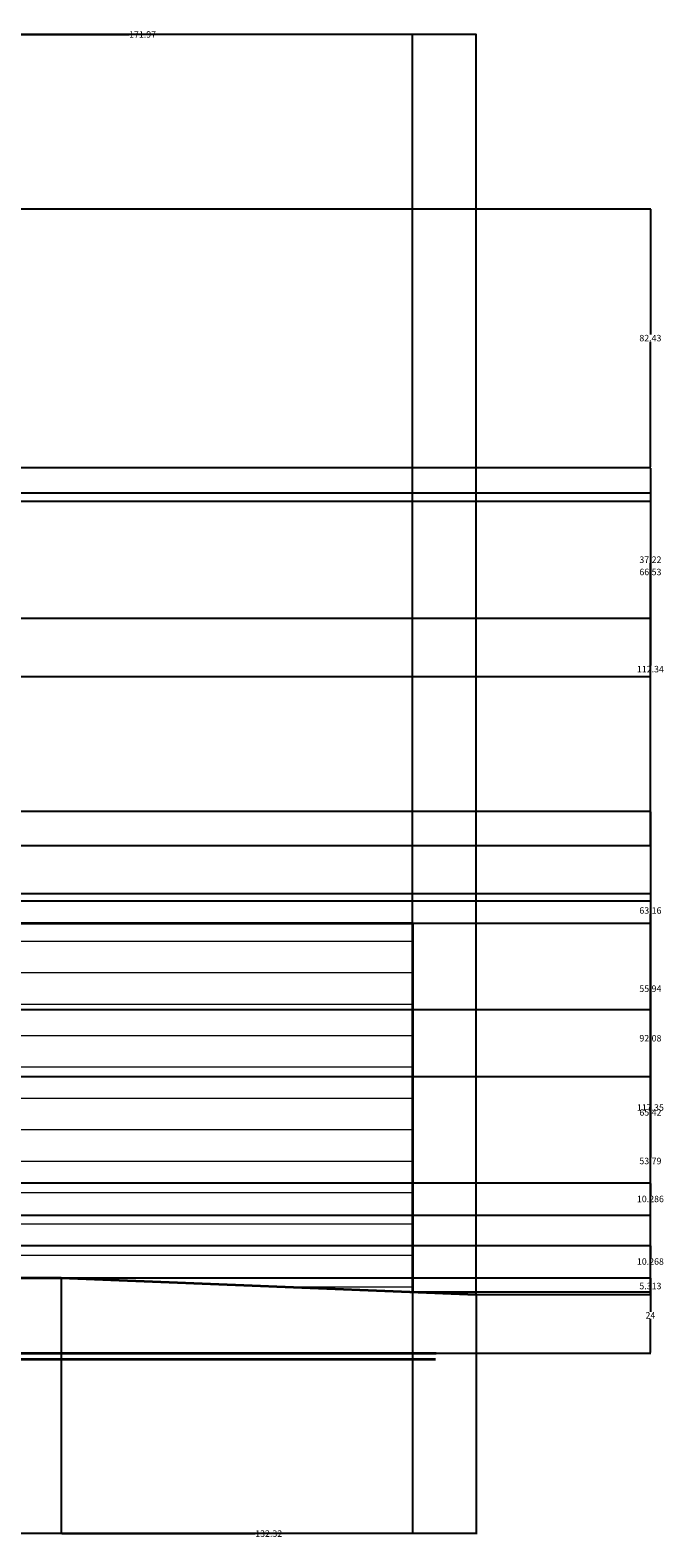
# Model space of a CAD drawing. Units: inches. Extents: x -30 to 1188, y 40 to 520.
# Tile 7 of 7: x 986 to 1188, y 40 to 520. Entities that reach past the tile are written whole.
import ezdxf

# ---------------------------------------------------------------- set-up
doc = ezdxf.new("R2010")
doc.units = ezdxf.units.IN
doc.header["$MEASUREMENT"] = 0
for name, color, linetype, lineweight in [('A-ANNO-DIMS', 2, 'Continuous', 18), ('A-ELEV', 7, 'Continuous', 35), ('A-ELEV-PATT', 8, 'Continuous', 13)]:
    doc.layers.add(name, color=color, linetype=linetype, lineweight=lineweight)
doc.styles.get("Standard").update_dxf_attribs({"font": 'arial.ttf'})
doc.dimstyles.get("Standard").update_dxf_attribs({"dimtxt": 2.0625, "dimasz": 0.18, "dimexe": 0.18, "dimexo": 0.0625, "dimgap": 0.09, "dimtad": 0, "dimtih": 1, "dimtoh": 1, "dimdec": 4, "dimzin": 0, "dimdsep": 46, "dimlunit": 4, "dimtxsty": 'Standard', "dimcen": 0.09, "dimadec": 0, "dimazin": 0, "dimtfac": 1, "dimtdec": 4, "dimtofl": 0, "dimtmove": 0, "dimatfit": 3, "dimfxl": 1, "dimtolj": 1, "dimtzin": 0, "dimarcsym": 0})

# ---------------------------------------------------------------- blocks, each defined once
blk = doc.blocks.new('*D4')
at = {"layer": 'A-ANNO-DIMS', "color": 0, "lineweight": -2, "transparency": 16777216}
for p, q in [((73.66, 122.81), (73.66, 41.19)), ((1107.88, 118.31), (1107.88, 41.19)), ((73.84, 41.37), (586.5, 41.37)), ((1107.7, 41.37), (595.03, 41.37))]:
    blk.add_line(p, q, dxfattribs=at)
at = {"layer": 'A-ANNO-DIMS', "color": 0, "transparency": 16777216}
for points in [[(73.84, 41.4), (73.84, 41.34), (73.66, 41.37)], [(1107.7, 41.4), (1107.7, 41.34), (1107.88, 41.37)]]:
    blk.add_solid(points, dxfattribs=at)
at = {"layer": 'Defpoints', "color": 0, "transparency": 16777216}
for p in [(73.66, 122.87), (1107.88, 118.38), (1107.88, 41.37)]:
    blk.add_point(p, dxfattribs=at)
at = {"layer": 'A-ANNO-DIMS', "color": 0, "transparency": 16777216, "insert": (590.77, 41.37), "char_height": 2.062, "attachment_point": 5}
blk.add_mtext('\\A1;1034.2', dxfattribs=at)
blk = doc.blocks.new('*D8')
at = {"layer": 'A-ANNO-DIMS', "color": 0, "lineweight": -2, "transparency": 16777216}
for p, q in [((935.9, 235.79), (935.9, 518.97)), ((936.08, 518.79), (1017.62, 518.79)), ((1107.7, 518.79), (1026.16, 518.79)), ((1107.88, 235.79), (1107.88, 518.97))]:
    blk.add_line(p, q, dxfattribs=at)
at = {"layer": 'A-ANNO-DIMS', "color": 0, "transparency": 16777216}
for points in [[(936.08, 518.82), (936.08, 518.76), (935.9, 518.79)], [(1107.7, 518.82), (1107.7, 518.76), (1107.88, 518.79)]]:
    blk.add_solid(points, dxfattribs=at)
at = {"layer": 'Defpoints', "color": 0, "transparency": 16777216}
for p in [(1107.88, 518.79), (935.9, 235.73), (1107.88, 235.73)]:
    blk.add_point(p, dxfattribs=at)
at = {"layer": 'A-ANNO-DIMS', "color": 0, "transparency": 16777216, "insert": (1021.89, 518.79), "char_height": 2.062, "attachment_point": 5}
blk.add_mtext('\\A1;171.97', dxfattribs=at)
blk = doc.blocks.new('*D19')
at = {"layer": 'A-ANNO-DIMS', "color": 0, "lineweight": -2, "transparency": 16777216}
for p, q in [((1107.94, 235.73), (1183.93, 235.73)), ((1183.75, 235.55), (1183.75, 178.2)), ((1183.75, 118.56), (1183.75, 175.91)), ((1107.94, 118.38), (1183.93, 118.38))]:
    blk.add_line(p, q, dxfattribs=at)
at = {"layer": 'A-ANNO-DIMS', "color": 0, "transparency": 16777216}
for points in [[(1183.72, 235.55), (1183.78, 235.55), (1183.75, 235.73)], [(1183.72, 118.56), (1183.78, 118.56), (1183.75, 118.38)]]:
    blk.add_solid(points, dxfattribs=at)
at = {"layer": 'Defpoints', "color": 0, "transparency": 16777216}
for p in [(1107.88, 235.73), (1183.75, 235.73), (1107.88, 118.38)]:
    blk.add_point(p, dxfattribs=at)
at = {"layer": 'A-ANNO-DIMS', "color": 0, "transparency": 16777216, "insert": (1183.75, 177.05), "char_height": 2.062, "attachment_point": 5}
blk.add_mtext('\\A1;117.35', dxfattribs=at)
blk = doc.blocks.new('*D23')
at = {"layer": 'A-ANNO-DIMS', "color": 0, "lineweight": -2, "transparency": 16777216}
for p, q in [((980.79, 372.83), (1183.93, 372.83)), ((1183.75, 372.65), (1183.75, 317.8)), ((1183.75, 260.67), (1183.75, 315.52)), ((980.79, 260.49), (1183.93, 260.49))]:
    blk.add_line(p, q, dxfattribs=at)
at = {"layer": 'A-ANNO-DIMS', "color": 0, "transparency": 16777216}
for points in [[(1183.72, 372.65), (1183.78, 372.65), (1183.75, 372.83)], [(1183.72, 260.67), (1183.78, 260.67), (1183.75, 260.49)]]:
    blk.add_solid(points, dxfattribs=at)
at = {"layer": 'Defpoints', "color": 0, "transparency": 16777216}
for p in [(980.73, 372.83), (1183.75, 372.83), (980.73, 260.49)]:
    blk.add_point(p, dxfattribs=at)
at = {"layer": 'A-ANNO-DIMS', "color": 0, "transparency": 16777216, "insert": (1183.75, 316.66), "char_height": 2.062, "attachment_point": 5}
blk.add_mtext('\\A1;112.34', dxfattribs=at)
blk = doc.blocks.new('*D26')
at = {"layer": 'A-ANNO-DIMS', "color": 0, "lineweight": -2, "transparency": 16777216}
for p, q in [((798.37, 380.86), (1183.93, 380.86)), ((1183.75, 380.68), (1183.75, 348.74)), ((1183.75, 314.51), (1183.75, 346.45)), ((798.37, 314.33), (1183.93, 314.33))]:
    blk.add_line(p, q, dxfattribs=at)
at = {"layer": 'A-ANNO-DIMS', "color": 0, "transparency": 16777216}
for points in [[(1183.72, 380.68), (1183.78, 380.68), (1183.75, 380.86)], [(1183.72, 314.51), (1183.78, 314.51), (1183.75, 314.33)]]:
    blk.add_solid(points, dxfattribs=at)
at = {"layer": 'Defpoints', "color": 0, "transparency": 16777216}
for p in [(798.3, 380.86), (1183.75, 380.86), (798.3, 314.33)]:
    blk.add_point(p, dxfattribs=at)
at = {"layer": 'A-ANNO-DIMS', "color": 0, "transparency": 16777216, "insert": (1183.75, 347.6), "char_height": 2.062, "attachment_point": 5}
blk.add_mtext('\\A1;66.53', dxfattribs=at)
blk = doc.blocks.new('*D30')
at = {"layer": 'A-ANNO-DIMS', "color": 0, "lineweight": -2, "transparency": 16777216}
for p, q in [((935.97, 463.29), (1183.93, 463.29)), ((1183.75, 463.11), (1183.75, 423.22)), ((1183.75, 381.04), (1183.75, 420.93)), ((798.37, 380.86), (1183.93, 380.86))]:
    blk.add_line(p, q, dxfattribs=at)
at = {"layer": 'A-ANNO-DIMS', "color": 0, "transparency": 16777216}
for points in [[(1183.72, 463.11), (1183.78, 463.11), (1183.75, 463.29)], [(1183.72, 381.04), (1183.78, 381.04), (1183.75, 380.86)]]:
    blk.add_solid(points, dxfattribs=at)
at = {"layer": 'Defpoints', "color": 0, "transparency": 16777216}
for p in [(935.9, 463.29), (1183.75, 463.29), (798.3, 380.86)]:
    blk.add_point(p, dxfattribs=at)
at = {"layer": 'A-ANNO-DIMS', "color": 0, "transparency": 16777216, "insert": (1183.75, 422.08), "char_height": 2.062, "attachment_point": 5}
blk.add_mtext('\\A1;82.43', dxfattribs=at)
blk = doc.blocks.new('*D35')
at = {"layer": 'A-ANNO-DIMS', "color": 0, "lineweight": -2, "transparency": 16777216}
for p, q in [((99.49, 122.87), (1183.93, 122.87)), ((1183.75, 122.69), (1183.75, 112)), ((1183.75, 99.05), (1183.75, 109.75)), ((99.49, 98.87), (1183.93, 98.87))]:
    blk.add_line(p, q, dxfattribs=at)
at = {"layer": 'A-ANNO-DIMS', "color": 0, "transparency": 16777216}
for points in [[(1183.72, 122.69), (1183.78, 122.69), (1183.75, 122.87)], [(1183.72, 99.05), (1183.78, 99.05), (1183.75, 98.87)]]:
    blk.add_solid(points, dxfattribs=at)
at = {"layer": 'Defpoints', "color": 0, "transparency": 16777216}
for p in [(99.43, 122.87), (1183.75, 122.87), (99.43, 98.87)]:
    blk.add_point(p, dxfattribs=at)
at = {"layer": 'A-ANNO-DIMS', "color": 0, "transparency": 16777216, "insert": (1183.75, 110.87), "char_height": 2.062, "attachment_point": 5}
blk.add_mtext('\\A1;24', dxfattribs=at)
blk = doc.blocks.new('*D36')
at = {"layer": 'A-ANNO-DIMS', "color": 0, "lineweight": -2, "transparency": 16777216}
for p, q in [((99.49, 133.14), (1183.93, 133.14)), ((1183.75, 132.96), (1183.75, 129.15)), ((1183.75, 123.05), (1183.75, 126.86)), ((99.49, 122.87), (1183.93, 122.87))]:
    blk.add_line(p, q, dxfattribs=at)
at = {"layer": 'A-ANNO-DIMS', "color": 0, "transparency": 16777216}
for points in [[(1183.72, 132.96), (1183.78, 132.96), (1183.75, 133.14)], [(1183.72, 123.05), (1183.78, 123.05), (1183.75, 122.87)]]:
    blk.add_solid(points, dxfattribs=at)
at = {"layer": 'Defpoints', "color": 0, "transparency": 16777216}
for p in [(99.43, 133.14), (1183.75, 133.14), (99.43, 122.87)]:
    blk.add_point(p, dxfattribs=at)
at = {"layer": 'A-ANNO-DIMS', "color": 0, "transparency": 16777216, "insert": (1183.75, 128.01), "char_height": 2.062, "attachment_point": 5}
blk.add_mtext('\\A1;10.268', dxfattribs=at)
blk = doc.blocks.new('*D37')
at = {"layer": 'A-ANNO-DIMS', "color": 0, "lineweight": -2, "transparency": 16777216}
for p, q in [((99.49, 186.93), (1183.93, 186.93)), ((1183.75, 186.75), (1183.75, 161.18)), ((1183.75, 133.32), (1183.75, 158.89)), ((99.49, 133.14), (1183.93, 133.14))]:
    blk.add_line(p, q, dxfattribs=at)
at = {"layer": 'A-ANNO-DIMS', "color": 0, "transparency": 16777216}
for points in [[(1183.72, 186.75), (1183.78, 186.75), (1183.75, 186.93)], [(1183.72, 133.32), (1183.78, 133.32), (1183.75, 133.14)]]:
    blk.add_solid(points, dxfattribs=at)
at = {"layer": 'Defpoints', "color": 0, "transparency": 16777216}
for p in [(99.43, 186.93), (1183.75, 186.93), (99.43, 133.14)]:
    blk.add_point(p, dxfattribs=at)
at = {"layer": 'A-ANNO-DIMS', "color": 0, "transparency": 16777216, "insert": (1183.75, 160.03), "char_height": 2.062, "attachment_point": 5}
blk.add_mtext('\\A1;53.79', dxfattribs=at)
blk = doc.blocks.new('*D38')
at = {"layer": 'A-ANNO-DIMS', "color": 0, "lineweight": -2, "transparency": 16777216}
for p, q in [((99.49, 242.87), (1183.93, 242.87)), ((1183.75, 242.69), (1183.75, 216.04)), ((1183.75, 187.11), (1183.75, 213.76)), ((99.49, 186.93), (1183.93, 186.93))]:
    blk.add_line(p, q, dxfattribs=at)
at = {"layer": 'A-ANNO-DIMS', "color": 0, "transparency": 16777216}
for points in [[(1183.72, 242.69), (1183.78, 242.69), (1183.75, 242.87)], [(1183.72, 187.11), (1183.78, 187.11), (1183.75, 186.93)]]:
    blk.add_solid(points, dxfattribs=at)
at = {"layer": 'Defpoints', "color": 0, "transparency": 16777216}
for p in [(99.43, 242.87), (1183.75, 242.87), (99.43, 186.93)]:
    blk.add_point(p, dxfattribs=at)
at = {"layer": 'A-ANNO-DIMS', "color": 0, "transparency": 16777216, "insert": (1183.75, 214.9), "char_height": 2.062, "attachment_point": 5}
blk.add_mtext('\\A1;55.94', dxfattribs=at)
blk = doc.blocks.new('*D39')
at = {"layer": 'A-ANNO-DIMS', "color": 0, "lineweight": -2, "transparency": 16777216}
for p, q in [((358.49, 186.93), (1183.93, 186.93)), ((1183.75, 186.75), (1183.75, 161.18)), ((1183.75, 133.32), (1183.75, 158.89)), ((358.49, 133.14), (1183.93, 133.14))]:
    blk.add_line(p, q, dxfattribs=at)
at = {"layer": 'A-ANNO-DIMS', "color": 0, "transparency": 16777216}
for points in [[(1183.72, 186.75), (1183.78, 186.75), (1183.75, 186.93)], [(1183.72, 133.32), (1183.78, 133.32), (1183.75, 133.14)]]:
    blk.add_solid(points, dxfattribs=at)
at = {"layer": 'Defpoints', "color": 0, "transparency": 16777216}
for p in [(358.42, 186.93), (1183.75, 186.93), (358.42, 133.14)]:
    blk.add_point(p, dxfattribs=at)
at = {"layer": 'A-ANNO-DIMS', "color": 0, "transparency": 16777216, "insert": (1183.75, 160.03), "char_height": 2.062, "attachment_point": 5}
blk.add_mtext('\\A1;53.79', dxfattribs=at)
blk = doc.blocks.new('*D40')
at = {"layer": 'A-ANNO-DIMS', "color": 0, "lineweight": -2, "transparency": 16777216}
for p, q in [((358.49, 242.87), (1183.93, 242.87)), ((1183.75, 242.69), (1183.75, 216.04)), ((1183.75, 187.11), (1183.75, 213.76)), ((358.49, 186.93), (1183.93, 186.93))]:
    blk.add_line(p, q, dxfattribs=at)
at = {"layer": 'A-ANNO-DIMS', "color": 0, "transparency": 16777216}
for points in [[(1183.72, 242.69), (1183.78, 242.69), (1183.75, 242.87)], [(1183.72, 187.11), (1183.78, 187.11), (1183.75, 186.93)]]:
    blk.add_solid(points, dxfattribs=at)
at = {"layer": 'Defpoints', "color": 0, "transparency": 16777216}
for p in [(358.42, 242.87), (1183.75, 242.87), (358.42, 186.93)]:
    blk.add_point(p, dxfattribs=at)
at = {"layer": 'A-ANNO-DIMS', "color": 0, "transparency": 16777216, "insert": (1183.75, 214.9), "char_height": 2.062, "attachment_point": 5}
blk.add_mtext('\\A1;55.94', dxfattribs=at)
blk = doc.blocks.new('*D48')
at = {"layer": 'A-ANNO-DIMS', "color": 0, "lineweight": -2, "transparency": 16777216}
for p, q in [((995.92, 122.81), (995.92, 41.19)), ((1128.25, 117.5), (1128.25, 41.19)), ((996.1, 41.37), (1057.82, 41.37)), ((1128.07, 41.37), (1066.35, 41.37))]:
    blk.add_line(p, q, dxfattribs=at)
at = {"layer": 'A-ANNO-DIMS', "color": 0, "transparency": 16777216}
for points in [[(996.1, 41.4), (996.1, 41.34), (995.92, 41.37)], [(1128.07, 41.4), (1128.07, 41.34), (1128.25, 41.37)]]:
    blk.add_solid(points, dxfattribs=at)
at = {"layer": 'Defpoints', "color": 0, "transparency": 16777216}
for p in [(995.92, 122.87), (1128.25, 117.56), (1128.25, 41.37)]:
    blk.add_point(p, dxfattribs=at)
at = {"layer": 'A-ANNO-DIMS', "color": 0, "transparency": 16777216, "insert": (1062.09, 41.37), "char_height": 2.062, "attachment_point": 5}
blk.add_mtext('\\A1;132.32', dxfattribs=at)
blk = doc.blocks.new('*D49')
at = {"layer": 'A-ANNO-DIMS', "color": 0, "lineweight": -2, "transparency": 16777216}
for p, q in [((995.99, 122.87), (1183.93, 122.87)), ((1183.75, 122.69), (1183.75, 121.36)), ((1128.31, 117.56), (1183.93, 117.56)), ((1183.75, 117.74), (1183.75, 119.07))]:
    blk.add_line(p, q, dxfattribs=at)
at = {"layer": 'A-ANNO-DIMS', "color": 0, "transparency": 16777216}
for points in [[(1183.72, 122.69), (1183.78, 122.69), (1183.75, 122.87)], [(1183.72, 117.74), (1183.78, 117.74), (1183.75, 117.56)]]:
    blk.add_solid(points, dxfattribs=at)
at = {"layer": 'Defpoints', "color": 0, "transparency": 16777216}
for p in [(995.92, 122.87), (1128.25, 117.56), (1183.75, 117.56)]:
    blk.add_point(p, dxfattribs=at)
at = {"layer": 'A-ANNO-DIMS', "color": 0, "transparency": 16777216, "insert": (1183.75, 120.22), "char_height": 2.062, "attachment_point": 5}
blk.add_mtext('\\A1;5.313', dxfattribs=at)
blk = doc.blocks.new('*D61')
at = {"layer": 'A-ANNO-DIMS', "color": 0, "lineweight": -2, "transparency": 16777216}
for p, q in [((653.09, 208.22), (1183.93, 208.22)), ((1183.75, 208.04), (1183.75, 176.65)), ((1183.75, 142.98), (1183.75, 174.36)), ((652.92, 142.8), (1183.93, 142.8))]:
    blk.add_line(p, q, dxfattribs=at)
at = {"layer": 'A-ANNO-DIMS', "color": 0, "transparency": 16777216}
for points in [[(1183.72, 208.04), (1183.78, 208.04), (1183.75, 208.22)], [(1183.72, 142.98), (1183.78, 142.98), (1183.75, 142.8)]]:
    blk.add_solid(points, dxfattribs=at)
at = {"layer": 'Defpoints', "color": 0, "transparency": 16777216}
for p in [(653.03, 208.22), (1183.75, 208.22), (652.86, 142.8)]:
    blk.add_point(p, dxfattribs=at)
at = {"layer": 'A-ANNO-DIMS', "color": 0, "transparency": 16777216, "insert": (1183.75, 175.51), "char_height": 2.062, "attachment_point": 5}
blk.add_mtext('\\A1;65.42', dxfattribs=at)
blk = doc.blocks.new('*D62')
at = {"layer": 'A-ANNO-DIMS', "color": 0, "lineweight": -2, "transparency": 16777216}
for p, q in [((652.92, 271.38), (1183.93, 271.38)), ((1183.75, 271.2), (1183.75, 240.94)), ((1183.75, 208.4), (1183.75, 238.65)), ((653.09, 208.22), (1183.93, 208.22))]:
    blk.add_line(p, q, dxfattribs=at)
at = {"layer": 'A-ANNO-DIMS', "color": 0, "transparency": 16777216}
for points in [[(1183.72, 271.2), (1183.78, 271.2), (1183.75, 271.38)], [(1183.72, 208.4), (1183.78, 208.4), (1183.75, 208.22)]]:
    blk.add_solid(points, dxfattribs=at)
at = {"layer": 'Defpoints', "color": 0, "transparency": 16777216}
for p in [(652.86, 271.38), (1183.75, 271.38), (653.03, 208.22)]:
    blk.add_point(p, dxfattribs=at)
at = {"layer": 'A-ANNO-DIMS', "color": 0, "transparency": 16777216, "insert": (1183.75, 239.8), "char_height": 2.062, "attachment_point": 5}
blk.add_mtext('\\A1;63.16', dxfattribs=at)
blk = doc.blocks.new('*D63')
at = {"layer": 'A-ANNO-DIMS', "color": 0, "lineweight": -2, "transparency": 16777216}
for p, q in [((576.85, 153.08), (1183.93, 153.08)), ((1183.75, 152.9), (1183.75, 149.08)), ((1183.75, 142.98), (1183.75, 146.8)), ((588.03, 142.8), (1183.93, 142.8))]:
    blk.add_line(p, q, dxfattribs=at)
at = {"layer": 'A-ANNO-DIMS', "color": 0, "transparency": 16777216}
for points in [[(1183.72, 152.9), (1183.78, 152.9), (1183.75, 153.08)], [(1183.72, 142.98), (1183.78, 142.98), (1183.75, 142.8)]]:
    blk.add_solid(points, dxfattribs=at)
at = {"layer": 'Defpoints', "color": 0, "transparency": 16777216}
for p in [(576.78, 153.08), (587.97, 142.8), (1183.75, 142.8)]:
    blk.add_point(p, dxfattribs=at)
at = {"layer": 'A-ANNO-DIMS', "color": 0, "transparency": 16777216, "insert": (1183.75, 147.94), "char_height": 2.062, "attachment_point": 5}
blk.add_mtext('\\A1;10.286', dxfattribs=at)
blk = doc.blocks.new('*D64')
at = {"layer": 'A-ANNO-DIMS', "color": 0, "lineweight": -2, "transparency": 16777216}
for p, q in [((576.85, 245.17), (1183.93, 245.17)), ((1183.75, 244.99), (1183.75, 200.27)), ((1183.75, 153.26), (1183.75, 197.98)), ((576.85, 153.08), (1183.93, 153.08))]:
    blk.add_line(p, q, dxfattribs=at)
at = {"layer": 'A-ANNO-DIMS', "color": 0, "transparency": 16777216}
for points in [[(1183.72, 244.99), (1183.78, 244.99), (1183.75, 245.17)], [(1183.72, 153.26), (1183.78, 153.26), (1183.75, 153.08)]]:
    blk.add_solid(points, dxfattribs=at)
at = {"layer": 'Defpoints', "color": 0, "transparency": 16777216}
for p in [(576.78, 245.17), (1183.75, 245.17), (576.78, 153.08)]:
    blk.add_point(p, dxfattribs=at)
at = {"layer": 'A-ANNO-DIMS', "color": 0, "transparency": 16777216, "insert": (1183.75, 199.12), "char_height": 2.062, "attachment_point": 5}
blk.add_mtext('\\A1;92.08', dxfattribs=at)
blk = doc.blocks.new('*D68')
at = {"layer": 'A-ANNO-DIMS', "color": 0, "lineweight": -2, "transparency": 16777216}
for p, q in [((580.04, 370.13), (1183.93, 370.13)), ((1183.75, 369.95), (1183.75, 352.67)), ((1183.75, 333.09), (1183.75, 350.38)), ((580.04, 332.91), (1183.93, 332.91))]:
    blk.add_line(p, q, dxfattribs=at)
at = {"layer": 'A-ANNO-DIMS', "color": 0, "transparency": 16777216}
for points in [[(1183.72, 369.95), (1183.78, 369.95), (1183.75, 370.13)], [(1183.72, 333.09), (1183.78, 333.09), (1183.75, 332.91)]]:
    blk.add_solid(points, dxfattribs=at)
at = {"layer": 'Defpoints', "color": 0, "transparency": 16777216}
for p in [(579.97, 370.13), (1183.75, 370.13), (579.97, 332.91)]:
    blk.add_point(p, dxfattribs=at)
at = {"layer": 'A-ANNO-DIMS', "color": 0, "transparency": 16777216, "insert": (1183.75, 351.52), "char_height": 2.062, "attachment_point": 5}
blk.add_mtext('\\A1;37.22', dxfattribs=at)
blk = doc.blocks.new('*D74')
at = {"layer": 'A-ANNO-DIMS', "color": 0, "lineweight": -2, "transparency": 16777216}
for p, q in [((30.14, 98.93), (30.14, 518.97)), ((30.32, 518.79), (574.32, 518.79)), ((1128.07, 518.79), (584.07, 518.79)), ((1128.25, 117.62), (1128.25, 518.97))]:
    blk.add_line(p, q, dxfattribs=at)
at = {"layer": 'A-ANNO-DIMS', "color": 0, "transparency": 16777216}
for points in [[(30.32, 518.82), (30.32, 518.76), (30.14, 518.79)], [(1128.07, 518.82), (1128.07, 518.76), (1128.25, 518.79)]]:
    blk.add_solid(points, dxfattribs=at)
at = {"layer": 'Defpoints', "color": 0, "transparency": 16777216}
for p in [(1128.25, 518.79), (1128.25, 117.56), (30.14, 98.87)]:
    blk.add_point(p, dxfattribs=at)
at = {"layer": 'A-ANNO-DIMS', "color": 0, "transparency": 16777216, "insert": (579.19, 518.79), "char_height": 2.0625, "attachment_point": 5}
blk.add_mtext('\\A1;1098.11', dxfattribs=at)

msp = doc.modelspace()

# ---------------------------------------------------------------- hatches: boundary and pattern name
at = {"layer": 'A-ELEV-PATT'}
h = msp.add_hatch(dxfattribs=at)
h.set_pattern_fill('ANSI31', color=256, scale=80, angle=135)
h.paths.add_polyline_path([(1107.8751, 235.7299), (935.904, 235.7299), (935.904, 122.8714), (995.9226, 122.8714), (1107.8751, 118.3767)])

# ---------------------------------------------------------------- linework, layer by layer
at = {"layer": 'A-ELEV'}
for p, q in [((935.904, 235.7299), (1107.8751, 235.7299)), ((1107.8751, 235.7299), (1107.8751, 118.3767)), ((935.904, 122.8714), (995.9226, 122.8714)), ((995.9226, 122.8714), (1128.2474, 117.5588)), ((799.1412, 96.8714), (1115.2418, 96.8714)), ((799.4646, 98.8714), (1115.4196, 98.8714))]:
    msp.add_line(p, q, dxfattribs=at)

# ---------------------------------------------------------------- dimensions: what is measured, and where the dimension line sits
at = {"layer": 'A-ANNO-DIMS'}
for base, p1, p2, override, picture, middle in [((1128.2474, 518.7934), (30.1395, 98.8714), (1128.2474, 117.5588), {"dimdec": 2, "dimlfac": 1, "dimrnd": 0, "dimzin": 0, "dimdsep": 46, "dimlunit": 2}, '*D74', (579.1935, 518.7934)), ((1107.8751, 518.7934), (935.904, 235.7299), (1107.8751, 235.7299), {"dimdec": 2, "dimlfac": 1, "dimrnd": 0, "dimzin": 0, "dimdsep": 46, "dimlunit": 2}, '*D8', (1021.8896, 518.7934)), ((1107.8751, 41.3714), (73.6582, 122.8714), (1107.8751, 118.3767), {"dimdec": 1, "dimlfac": 1, "dimrnd": 0, "dimzin": 0, "dimdsep": 46, "dimlunit": 2}, '*D4', (590.7666, 41.3714)), ((1128.2474, 41.3714), (995.9226, 122.8714), (1128.2474, 117.5588), {"dimdec": 2, "dimlfac": 1, "dimrnd": 0, "dimzin": 0, "dimdsep": 46, "dimlunit": 2}, '*D48', (1062.085, 41.3714))]:
    dim = msp.add_linear_dim(base=base, p1=p1, p2=p2, dimstyle='Standard', override=override, dxfattribs=at)
    dim.commit()
    dim.dimension.update_dxf_attribs({"geometry": picture, "text_midpoint": middle})
for base, p1, p2, override, picture, middle in [((1183.7474, 463.2934), (798.3036, 380.8615), (935.904, 463.2934), {"dimdec": 2, "dimlfac": 1, "dimrnd": 0, "dimzin": 0, "dimdsep": 46, "dimlunit": 2}, '*D30', (1183.7474, 422.0775)), ((1183.7474, 380.8615), (798.3036, 314.3348), (798.3036, 380.8615), {"dimdec": 2, "dimlfac": 1, "dimrnd": 0, "dimzin": 0, "dimdsep": 46, "dimlunit": 2}, '*D26', (1183.7474, 347.5982)), ((1183.7474, 370.1304), (579.9749, 332.9128), (579.9749, 370.1304), {"dimdec": 2, "dimlfac": 1, "dimrnd": 0, "dimzin": 0, "dimdsep": 46, "dimlunit": 2}, '*D68', (1183.7474, 351.5216)), ((1183.7474, 372.8284), (980.7252, 260.4906), (980.7252, 372.8284), {"dimdec": 2, "dimlfac": 1, "dimrnd": 0, "dimzin": 0, "dimdsep": 46, "dimlunit": 2}, '*D23', (1183.7474, 316.6595)), ((1183.7474, 271.3754), (653.0318, 208.218), (652.8622, 271.3754), {"dimdec": 2, "dimlfac": 1, "dimrnd": 0, "dimzin": 0, "dimdsep": 46, "dimlunit": 2}, '*D62', (1183.7474, 239.7967)), ((1183.7474, 245.1654), (576.7826, 153.0843), (576.7826, 245.1654), {"dimdec": 2, "dimlfac": 1, "dimrnd": 0, "dimzin": 0, "dimdsep": 46, "dimlunit": 2}, '*D64', (1183.7474, 199.1248)), ((1183.7474, 242.8714), (99.4312, 186.9265), (99.4312, 242.8714), {"dimdec": 2, "dimlfac": 1, "dimrnd": 0, "dimzin": 0, "dimdsep": 46, "dimlunit": 2}, '*D38', (1183.7474, 214.899)), ((1183.7474, 242.8714), (358.4247, 186.9265), (358.4247, 242.8714), {"dimdec": 2, "dimlfac": 1, "dimrnd": 0, "dimzin": 0, "dimdsep": 46, "dimlunit": 2}, '*D40', (1183.7474, 214.899)), ((1183.7474, 235.7299), (1107.8751, 118.3767), (1107.8751, 235.7299), {"dimdec": 2, "dimlfac": 1, "dimrnd": 0, "dimzin": 0, "dimdsep": 46, "dimlunit": 2}, '*D19', (1183.7474, 177.0533)), ((1183.7474, 208.218), (652.8622, 142.7981), (653.0318, 208.218), {"dimdec": 2, "dimlfac": 1, "dimrnd": 0, "dimzin": 0, "dimdsep": 46, "dimlunit": 2}, '*D61', (1183.7474, 175.508)), ((1183.7474, 186.9265), (99.4312, 133.1393), (99.4312, 186.9265), {"dimdec": 2, "dimlfac": 1, "dimrnd": 0, "dimzin": 0, "dimdsep": 46, "dimlunit": 2}, '*D37', (1183.7474, 160.0329)), ((1183.7474, 186.9265), (358.4247, 133.1393), (358.4247, 186.9265), {"dimdec": 2, "dimlfac": 1, "dimrnd": 0, "dimzin": 0, "dimdsep": 46, "dimlunit": 2}, '*D39', (1183.7474, 160.0329)), ((1183.7474, 142.7981), (576.7826, 153.0843), (587.9675, 142.7981), {"dimdec": 3, "dimlfac": 1, "dimrnd": 0, "dimzin": 0, "dimdsep": 46, "dimlunit": 2}, '*D63', (1183.7474, 147.9412)), ((1183.7474, 133.1393), (99.4312, 122.8714), (99.4312, 133.1393), {"dimdec": 3, "dimlfac": 1, "dimrnd": 0, "dimzin": 0, "dimdsep": 46, "dimlunit": 2}, '*D36', (1183.7474, 128.0054)), ((1183.7474, 122.8714), (99.4312, 98.8714), (99.4312, 122.8714), {"dimdec": 0, "dimlfac": 1, "dimrnd": 0, "dimzin": 0, "dimdsep": 46, "dimlunit": 2}, '*D35', (1183.7474, 110.8714)), ((1183.7474, 117.5588), (995.9226, 122.8714), (1128.2474, 117.5588), {"dimdec": 3, "dimlfac": 1, "dimrnd": 0, "dimzin": 0, "dimdsep": 46, "dimlunit": 2}, '*D49', (1183.7474, 120.2151))]:
    dim = msp.add_linear_dim(base=base, p1=p1, p2=p2, angle=90, dimstyle='Standard', override=override, dxfattribs=at)
    dim.commit()
    dim.dimension.update_dxf_attribs({"geometry": picture, "text_midpoint": middle})

doc.saveas('drawing.dxf')
